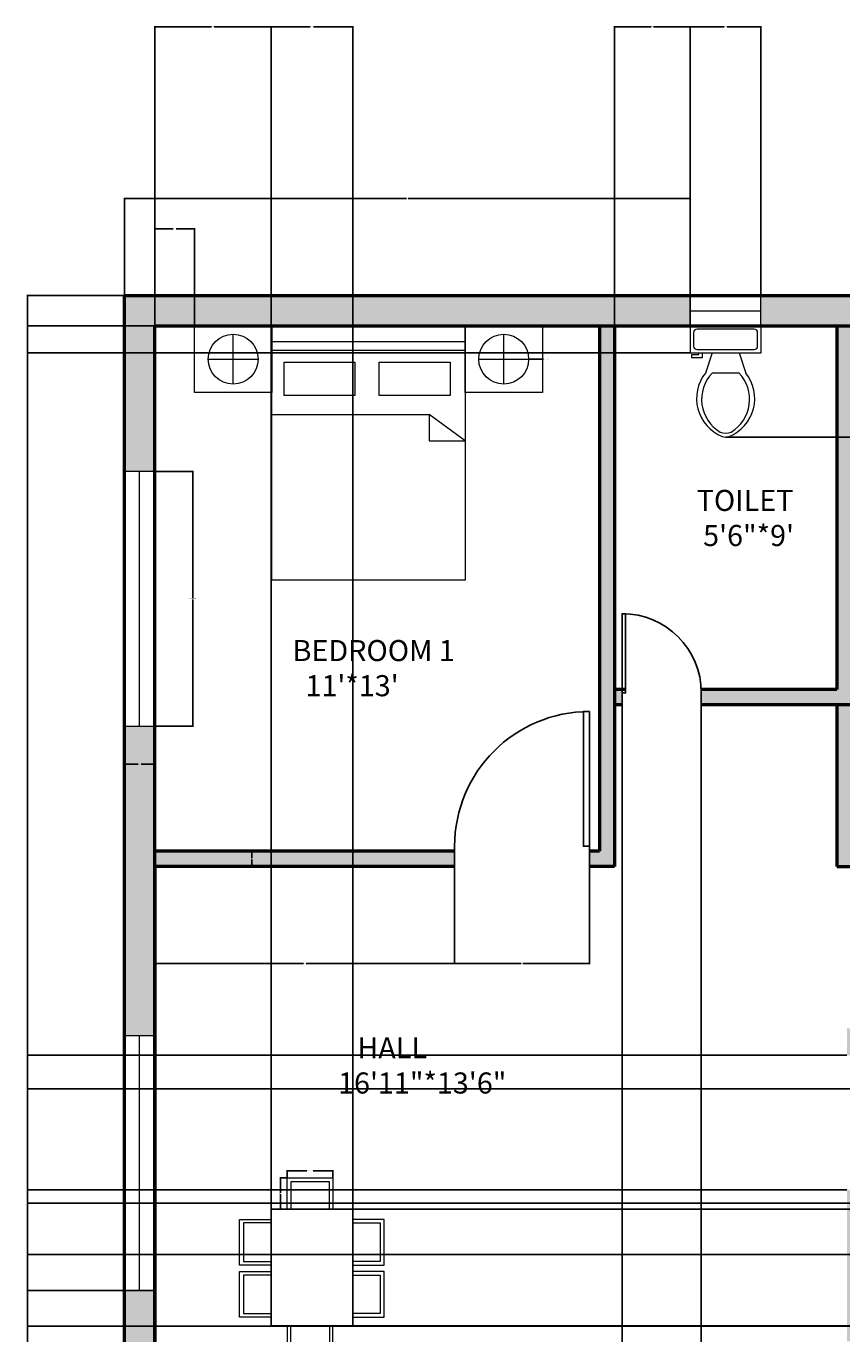
# Model space of a CAD drawing. Units: inches. Extents: x 2405 to 2823, y 1214 to 1813.
# Tile 3 of 4: x 2405 to 2647, y 1425 to 1813. Entities that reach past the tile are written whole.
import ezdxf

# ---------------------------------------------------------------- set-up
doc = ezdxf.new("R2010")
doc.units = ezdxf.units.IN
for name, color, linetype, lineweight in [('A-ANNO-DIMS', 2, 'Continuous', 18), ('A-AREA-IDEN', 30, 'Continuous', 25), ('A-FLOR-FIXT', 9, 'Continuous', 18), ('A-WALL-PATT', 252, 'Continuous', 13), ('DOOR', 133, 'Continuous', 25), ('FUR', 10, 'Continuous', 18), ('WALL', 140, 'Continuous', 50), ('WIND', 200, 'Continuous', 18)]:
    doc.layers.add(name, color=color, linetype=linetype, lineweight=lineweight)
doc.styles.get("Standard").update_dxf_attribs({"font": 'arial.ttf'})
doc.dimstyles.get("Standard").update_dxf_attribs({"dimtxt": 0.18, "dimasz": 0.18, "dimexe": 0.18, "dimexo": 0.0625, "dimgap": 0.09, "dimtad": 0, "dimtih": 1, "dimtoh": 1, "dimdec": 4, "dimzin": 0, "dimdsep": 46, "dimtxsty": 'Standard', "dimcen": 0.09, "dimadec": 0, "dimazin": 0, "dimtfac": 1, "dimtdec": 4, "dimtofl": 0, "dimtmove": 0, "dimatfit": 3, "dimfxl": 1, "dimtolj": 1, "dimtzin": 0, "dimarcsym": 0})

# ---------------------------------------------------------------- blocks, each defined once
blk = doc.blocks.new('*U2')
for p, q in [((0, 0), (0, -6)), ((40, 0), (40, -6))]:
    blk.add_line(p, q)
blk.add_lwpolyline([(0, 0), (0, 40), (1.75, 40), (1.75, 0)], close=True)
blk.add_arc((0, 0), 40, 0, 90)
blk = doc.blocks.new('*U4')
for p, q in [((9.5, -6), (9.5, -2)), ((-10, -8.5), (-8, -8.5)), ((-10, -9.5), (-10, -8.5)), ((-7, -9.5), (-10, -9.5)), ((-8, -8.5), (-8, -8)), ((-7, -8), (-7, -9.5)), ((-4, -8), (-6, -14)), ((4, -8), (6, -14)), ((4, -14), (-4, -14))]:
    blk.add_line(p, q)
blk.add_lwpolyline([(10.5, -8), (10.5, 0), (-10.5, 0), (-10.5, -8)], close=True)
for points in [[(-9.5, -2), (-9.5, -6)], [(8.5, -1), (-8.5, -1)], [(-8.5, -7), (8.5, -7)]]:
    blk.add_lwpolyline(points)
for centre, radius, start, end in [((-8.62, -1.88), 0.884, 81.8699, 188.1301), ((8.62, -1.88), 0.884, 351.8699, 98.1301), ((-8.62, -6.12), 0.884, 171.8699, 278.1301), ((8.62, -6.12), 0.884, 261.8699, 8.1301), ((3.52, -21.58), 12.17, 141.4691, 247.9714), ((4.2, -21.82), 11.33, 136.3677, 238.9468), ((-3.52, -21.58), 12.17, 292.0284, 38.5307), ((-4.2, -21.82), 11.33, 301.053, 43.6321), ((0, -27.88), 4, 245.7318, 294.2682), ((0, -29), 4, 254.8605, 285.1395)]:
    blk.add_arc(centre, radius, start, end)
blk = doc.blocks.new('BED-DOUBLE-WITH-NIGHTSTANDS')
for p, q in [((11.49, 58.17), (11.49, 72.97)), ((91.81, 58.17), (91.81, 72.97)), ((4.09, 65.57), (18.88, 65.57)), ((84.41, 65.57), (99.2, 65.57)), ((22.97, 49.14), (69.63, 49.14)), ((69.63, 49.14), (69.63, 41.32)), ((80.32, 41.32), (69.63, 49.14)), ((69.63, 41.32), (80.32, 41.32))]:
    blk.add_line(p, q)
for points in [[(0, 75.45), (22.97, 75.45), (22.97, 55.69), (0, 55.69)], [(22.97, 75.45), (80.32, 75.45), (80.32, 0), (22.97, 0)], [(80.32, 75.45), (103.29, 75.45), (103.29, 55.69), (80.32, 55.69)], [(22.97, 70.85), (80.32, 70.85), (80.32, 68.18), (22.97, 68.18)], [(26.59, 64.68), (47.64, 64.68), (47.64, 54.75), (26.59, 54.75)], [(54.85, 64.68), (75.89, 64.68), (75.89, 54.75), (54.85, 54.75)]]:
    blk.add_lwpolyline(points, close=True)
for centre in [(11.49, 65.57), (91.81, 65.57)]:
    blk.add_circle(centre, 7.4)
blk = doc.blocks.new('CHAIR-DINING')
for p, q in [((0, 0), (0, 9.36)), ((0, 9.36), (13.56, 9.36)), ((13.56, 9.36), (13.56, 0))]:
    blk.add_line(p, q)
blk.add_lwpolyline([(1.08, 0), (12.53, 0), (12.53, 8.17), (1.08, 8.17)], close=True)
blk = doc.blocks.new('WIN-75_625')
blk.add_line((4.5, 0), (4.5, 75.63))
blk.add_lwpolyline([(9, 75.63), (0, 75.63), (0, 0), (9, 0)], close=True)
blk = doc.blocks.new('*D12')
at = {"layer": 'A-ANNO-DIMS', "color": 0, "lineweight": -2, "transparency": 16777216}
for p, q in [((2482.12, 1471.1), (2482.12, 1473.25)), ((2482.3, 1473.07), (2487.95, 1473.07)), ((2495.5, 1473.07), (2489.85, 1473.07)), ((2495.68, 1471.1), (2495.68, 1473.25))]:
    blk.add_line(p, q, dxfattribs=at)
at = {"layer": 'A-ANNO-DIMS', "color": 0, "lineweight": 100, "transparency": 16777216}
for points in [[(2482.3, 1473.1), (2482.3, 1473.04), (2482.12, 1473.07)], [(2495.5, 1473.1), (2495.5, 1473.04), (2495.68, 1473.07)]]:
    blk.add_solid(points, dxfattribs=at)
at = {"layer": 'Defpoints', "color": 0, "lineweight": 100, "transparency": 16777216}
for p in [(2495.68, 1473.07), (2482.12, 1471.04), (2495.68, 1471.04)]:
    blk.add_point(p, dxfattribs=at)
at = {"layer": 'A-ANNO-DIMS', "color": 0, "transparency": 16777216, "insert": (2488.9, 1473.07), "char_height": 0.18, "attachment_point": 5}
blk.add_mtext('\\A1;CHAIR 14 TYP.', dxfattribs=at)
blk = doc.blocks.new('*D13')
at = {"layer": 'A-ANNO-DIMS', "color": 0, "lineweight": -2, "transparency": 16777216}
for p, q in [((2482.06, 1471.04), (2479.9, 1471.04)), ((2480.08, 1470.86), (2480.08, 1466.54)), ((2480.08, 1461.86), (2480.08, 1466.17)), ((2482.06, 1461.68), (2479.9, 1461.68))]:
    blk.add_line(p, q, dxfattribs=at)
at = {"layer": 'A-ANNO-DIMS', "color": 0, "lineweight": 100, "transparency": 16777216}
for points in [[(2480.05, 1470.86), (2480.11, 1470.86), (2480.08, 1471.04)], [(2480.05, 1461.86), (2480.11, 1461.86), (2480.08, 1461.68)]]:
    blk.add_solid(points, dxfattribs=at)
at = {"layer": 'Defpoints', "color": 0, "lineweight": 100, "transparency": 16777216}
for p in [(2480.08, 1471.04), (2482.12, 1471.04), (2482.12, 1461.68)]:
    blk.add_point(p, dxfattribs=at)
at = {"layer": 'A-ANNO-DIMS', "color": 0, "transparency": 16777216, "insert": (2480.08, 1466.36), "char_height": 0.18, "attachment_point": 5}
blk.add_mtext('\\A1;9 TYP.', dxfattribs=at)
blk = doc.blocks.new('*D18')
at = {"layer": 'A-ANNO-DIMS', "color": 0, "lineweight": -2, "transparency": 16777216}
for p, q in [((2442.83, 1680.74), (2454.29, 1680.74)), ((2454.11, 1680.56), (2454.11, 1643.11)), ((2454.11, 1605.29), (2454.11, 1642.74)), ((2442.83, 1605.11), (2454.29, 1605.11))]:
    blk.add_line(p, q, dxfattribs=at)
at = {"layer": 'A-ANNO-DIMS', "color": 0, "lineweight": 100, "transparency": 16777216}
for points in [[(2454.08, 1680.56), (2454.14, 1680.56), (2454.11, 1680.74)], [(2454.08, 1605.29), (2454.14, 1605.29), (2454.11, 1605.11)]]:
    blk.add_solid(points, dxfattribs=at)
at = {"layer": 'Defpoints', "color": 0, "lineweight": 100, "transparency": 16777216}
for p in [(2442.77, 1680.74), (2454.11, 1680.74), (2442.77, 1605.11)]:
    blk.add_point(p, dxfattribs=at)
at = {"layer": 'A-ANNO-DIMS', "color": 0, "transparency": 16777216, "insert": (2454.11, 1642.92), "char_height": 0.18, "attachment_point": 5}
blk.add_mtext('\\A1;WINDOW 76 TYP.', dxfattribs=at)
blk = doc.blocks.new('*D19')
at = {"layer": 'A-ANNO-DIMS', "color": 0, "lineweight": -2, "transparency": 16777216}
for p, q in [((2433.77, 1605.05), (2433.77, 1593.59)), ((2442.77, 1605.05), (2442.77, 1593.59)), ((2433.95, 1593.77), (2437.81, 1593.77)), ((2442.59, 1593.77), (2438.73, 1593.77))]:
    blk.add_line(p, q, dxfattribs=at)
at = {"layer": 'A-ANNO-DIMS', "color": 0, "lineweight": 100, "transparency": 16777216}
for points in [[(2433.95, 1593.8), (2433.95, 1593.74), (2433.77, 1593.77)], [(2442.59, 1593.8), (2442.59, 1593.74), (2442.77, 1593.77)]]:
    blk.add_solid(points, dxfattribs=at)
at = {"layer": 'Defpoints', "color": 0, "lineweight": 100, "transparency": 16777216}
for p in [(2433.77, 1605.11), (2442.77, 1605.11), (2442.77, 1593.77)]:
    blk.add_point(p, dxfattribs=at)
at = {"layer": 'A-ANNO-DIMS', "color": 0, "transparency": 16777216, "insert": (2438.27, 1593.77), "char_height": 0.18, "attachment_point": 5}
blk.add_mtext('\\A1;9 TYP.', dxfattribs=at)
blk = doc.blocks.new('*D23')
at = {"layer": 'A-ANNO-DIMS', "color": 0, "lineweight": -2, "transparency": 16777216}
for p, q in [((2433.71, 1732.93), (2404.79, 1732.93)), ((2404.97, 1732.75), (2404.97, 1488.61)), ((2404.97, 1244.11), (2404.97, 1488.25)), ((2586.21, 1243.93), (2404.79, 1243.93))]:
    blk.add_line(p, q, dxfattribs=at)
at = {"layer": 'A-ANNO-DIMS', "color": 0, "lineweight": 100, "transparency": 16777216}
for points in [[(2404.94, 1732.75), (2405, 1732.75), (2404.97, 1732.93)], [(2404.94, 1244.11), (2405, 1244.11), (2404.97, 1243.93)]]:
    blk.add_solid(points, dxfattribs=at)
at = {"layer": 'Defpoints', "color": 0, "lineweight": 100, "transparency": 16777216}
for p in [(2433.77, 1732.93), (2404.97, 1243.93), (2586.27, 1243.93)]:
    blk.add_point(p, dxfattribs=at)
at = {"layer": 'A-ANNO-DIMS', "color": 0, "transparency": 16777216, "insert": (2404.97, 1488.43), "char_height": 0.18, "attachment_point": 5}
blk.add_mtext('\\A1;489', dxfattribs=at)
blk = doc.blocks.new('*D25')
at = {"layer": 'A-ANNO-DIMS', "color": 0, "lineweight": -2, "transparency": 16777216}
for p, q in [((2442.71, 1437.52), (2404.79, 1437.52)), ((2404.97, 1437.34), (2404.97, 1419.66)), ((2404.97, 1401.61), (2404.97, 1419.29)), ((2442.71, 1401.43), (2404.79, 1401.43))]:
    blk.add_line(p, q, dxfattribs=at)
at = {"layer": 'A-ANNO-DIMS', "color": 0, "lineweight": 100, "transparency": 16777216}
for points in [[(2404.94, 1437.34), (2405, 1437.34), (2404.97, 1437.52)], [(2404.94, 1401.61), (2405, 1401.61), (2404.97, 1401.43)]]:
    blk.add_solid(points, dxfattribs=at)
at = {"layer": 'Defpoints', "color": 0, "lineweight": 100, "transparency": 16777216}
for p in [(2442.77, 1437.52), (2404.97, 1401.43), (2442.77, 1401.43)]:
    blk.add_point(p, dxfattribs=at)
at = {"layer": 'A-ANNO-DIMS', "color": 0, "transparency": 16777216, "insert": (2404.97, 1419.47), "char_height": 0.18, "attachment_point": 5}
blk.add_mtext('\\A1;36.09', dxfattribs=at)
blk = doc.blocks.new('*D32')
at = {"layer": 'A-ANNO-DIMS', "color": 0, "lineweight": -2, "transparency": 16777216}
for p, q in [((2433.77, 1732.99), (2433.77, 1761.91)), ((2433.95, 1761.73), (2517.49, 1761.73)), ((2601.59, 1761.73), (2518.05, 1761.73)), ((2601.77, 1732.99), (2601.77, 1761.91))]:
    blk.add_line(p, q, dxfattribs=at)
at = {"layer": 'A-ANNO-DIMS', "color": 0, "lineweight": 100, "transparency": 16777216}
for points in [[(2433.95, 1761.76), (2433.95, 1761.7), (2433.77, 1761.73)], [(2601.59, 1761.76), (2601.59, 1761.7), (2601.77, 1761.73)]]:
    blk.add_solid(points, dxfattribs=at)
at = {"layer": 'Defpoints', "color": 0, "lineweight": 100, "transparency": 16777216}
for p in [(2601.77, 1761.73), (2433.77, 1732.93), (2601.77, 1732.93)]:
    blk.add_point(p, dxfattribs=at)
at = {"layer": 'A-ANNO-DIMS', "color": 0, "transparency": 16777216, "insert": (2517.77, 1761.73), "char_height": 0.18, "attachment_point": 5}
blk.add_mtext('\\A1;168', dxfattribs=at)
blk = doc.blocks.new('*D33')
at = {"layer": 'A-ANNO-DIMS', "color": 0, "lineweight": -2, "transparency": 16777216}
for p, q in [((2601.77, 1732.99), (2601.77, 1812.91)), ((2601.95, 1812.73), (2611.8, 1812.73)), ((2622.58, 1812.73), (2612.73, 1812.73)), ((2622.76, 1732.99), (2622.76, 1812.91))]:
    blk.add_line(p, q, dxfattribs=at)
at = {"layer": 'A-ANNO-DIMS', "color": 0, "lineweight": 100, "transparency": 16777216}
for points in [[(2601.95, 1812.76), (2601.95, 1812.7), (2601.77, 1812.73)], [(2622.58, 1812.76), (2622.58, 1812.7), (2622.76, 1812.73)]]:
    blk.add_solid(points, dxfattribs=at)
at = {"layer": 'Defpoints', "color": 0, "lineweight": 100, "transparency": 16777216}
for p in [(2622.76, 1812.73), (2601.77, 1732.93), (2622.76, 1732.93)]:
    blk.add_point(p, dxfattribs=at)
at = {"layer": 'A-ANNO-DIMS', "color": 0, "transparency": 16777216, "insert": (2612.26, 1812.73), "char_height": 0.18, "attachment_point": 5}
blk.add_mtext('\\A1;20.987', dxfattribs=at)
blk = doc.blocks.new('*D41')
at = {"layer": 'A-ANNO-DIMS', "color": 0, "lineweight": -2, "transparency": 16777216}
for p, q in [((2648.21, 1507.39), (2404.79, 1507.39)), ((2404.97, 1507.21), (2404.97, 1487.57)), ((2404.97, 1467.57), (2404.97, 1487.21)), ((2648.21, 1467.39), (2404.79, 1467.39))]:
    blk.add_line(p, q, dxfattribs=at)
at = {"layer": 'A-ANNO-DIMS', "color": 0, "lineweight": 100, "transparency": 16777216}
for points in [[(2404.94, 1507.21), (2405, 1507.21), (2404.97, 1507.39)], [(2404.94, 1467.57), (2405, 1467.57), (2404.97, 1467.39)]]:
    blk.add_solid(points, dxfattribs=at)
at = {"layer": 'Defpoints', "color": 0, "lineweight": 100, "transparency": 16777216}
for p in [(2648.27, 1507.39), (2404.97, 1467.39), (2648.27, 1467.39)]:
    blk.add_point(p, dxfattribs=at)
at = {"layer": 'A-ANNO-DIMS', "color": 0, "transparency": 16777216, "insert": (2404.97, 1487.39), "char_height": 0.18, "attachment_point": 5}
blk.add_mtext('\\A1;40', dxfattribs=at)
blk = doc.blocks.new('*D42')
at = {"layer": 'A-ANNO-DIMS', "color": 0, "lineweight": -2, "transparency": 16777216}
for p, q in [((2605.03, 1615.87), (2605.03, 1214.95)), ((2581.53, 1614.9), (2581.53, 1214.95)), ((2581.71, 1215.13), (2592.95, 1215.13)), ((2604.85, 1215.13), (2593.61, 1215.13))]:
    blk.add_line(p, q, dxfattribs=at)
at = {"layer": 'A-ANNO-DIMS', "color": 0, "lineweight": 100, "transparency": 16777216}
for points in [[(2581.71, 1215.16), (2581.71, 1215.1), (2581.53, 1215.13)], [(2604.85, 1215.16), (2604.85, 1215.1), (2605.03, 1215.13)]]:
    blk.add_solid(points, dxfattribs=at)
at = {"layer": 'Defpoints', "color": 0, "lineweight": 100, "transparency": 16777216}
for p in [(2605.03, 1615.93), (2581.53, 1614.96), (2605.03, 1215.13)]:
    blk.add_point(p, dxfattribs=at)
at = {"layer": 'A-ANNO-DIMS', "color": 0, "transparency": 16777216, "insert": (2593.28, 1215.13), "char_height": 0.18, "attachment_point": 5}
blk.add_mtext('\\A1;23.5', dxfattribs=at)
blk = doc.blocks.new('*D44')
at = {"layer": 'A-ANNO-DIMS', "color": 0, "lineweight": -2, "transparency": 16777216}
for p, q in [((2477.3, 1427.08), (2477.3, 1812.91)), ((2477.48, 1812.73), (2488.96, 1812.73)), ((2501.38, 1812.73), (2489.89, 1812.73)), ((2501.56, 1427.08), (2501.56, 1812.91))]:
    blk.add_line(p, q, dxfattribs=at)
at = {"layer": 'A-ANNO-DIMS', "color": 0, "lineweight": 100, "transparency": 16777216}
for points in [[(2477.48, 1812.76), (2477.48, 1812.7), (2477.3, 1812.73)], [(2501.38, 1812.76), (2501.38, 1812.7), (2501.56, 1812.73)]]:
    blk.add_solid(points, dxfattribs=at)
at = {"layer": 'Defpoints', "color": 0, "lineweight": 100, "transparency": 16777216}
for p in [(2501.56, 1812.73), (2477.3, 1427.01), (2501.56, 1427.01)]:
    blk.add_point(p, dxfattribs=at)
at = {"layer": 'A-ANNO-DIMS', "color": 0, "transparency": 16777216, "insert": (2489.43, 1812.73), "char_height": 0.18, "attachment_point": 5}
blk.add_mtext('\\A1;24.266', dxfattribs=at)
blk = doc.blocks.new('*D45')
at = {"layer": 'A-ANNO-DIMS', "color": 0, "lineweight": -2, "transparency": 16777216}
for p, q in [((2477.36, 1461.68), (2822.75, 1461.68)), ((2822.57, 1461.5), (2822.57, 1444.53)), ((2822.57, 1427.19), (2822.57, 1444.16)), ((2477.36, 1427.01), (2822.75, 1427.01))]:
    blk.add_line(p, q, dxfattribs=at)
at = {"layer": 'A-ANNO-DIMS', "color": 0, "lineweight": 100, "transparency": 16777216}
for points in [[(2822.54, 1461.5), (2822.6, 1461.5), (2822.57, 1461.68)], [(2822.54, 1427.19), (2822.6, 1427.19), (2822.57, 1427.01)]]:
    blk.add_solid(points, dxfattribs=at)
at = {"layer": 'Defpoints', "color": 0, "lineweight": 100, "transparency": 16777216}
for p in [(2477.3, 1461.68), (2477.3, 1427.01), (2822.57, 1427.01)]:
    blk.add_point(p, dxfattribs=at)
at = {"layer": 'A-ANNO-DIMS', "color": 0, "transparency": 16777216, "insert": (2822.57, 1444.34), "char_height": 0.18, "attachment_point": 5}
blk.add_mtext('\\A1;34.66', dxfattribs=at)
blk = doc.blocks.new('*D47')
at = {"layer": 'A-ANNO-DIMS', "color": 0, "lineweight": -2, "transparency": 16777216}
for p, q in [((2763.89, 1497.45), (2404.79, 1497.45)), ((2404.97, 1497.27), (2404.97, 1480.64)), ((2404.97, 1463.65), (2404.97, 1480.28)), ((2763.89, 1463.47), (2404.79, 1463.47))]:
    blk.add_line(p, q, dxfattribs=at)
at = {"layer": 'A-ANNO-DIMS', "color": 0, "lineweight": 100, "transparency": 16777216}
for points in [[(2404.94, 1497.27), (2405, 1497.27), (2404.97, 1497.45)], [(2404.94, 1463.65), (2405, 1463.65), (2404.97, 1463.47)]]:
    blk.add_solid(points, dxfattribs=at)
at = {"layer": 'Defpoints', "color": 0, "lineweight": 100, "transparency": 16777216}
for p in [(2763.95, 1497.45), (2404.97, 1463.47), (2763.95, 1463.47)]:
    blk.add_point(p, dxfattribs=at)
at = {"layer": 'A-ANNO-DIMS', "color": 0, "transparency": 16777216, "insert": (2404.97, 1480.46), "char_height": 0.18, "attachment_point": 5}
blk.add_mtext('\\A1;33.98', dxfattribs=at)
blk = doc.blocks.new('*D49')
at = {"layer": 'A-ANNO-DIMS', "color": 0, "lineweight": -2, "transparency": 16777216}
for p, q in [((2442.77, 1401.49), (2442.77, 1812.91)), ((2442.95, 1812.73), (2459.64, 1812.73)), ((2477.12, 1812.73), (2460.43, 1812.73)), ((2477.3, 1427.08), (2477.3, 1812.91))]:
    blk.add_line(p, q, dxfattribs=at)
at = {"layer": 'A-ANNO-DIMS', "color": 0, "lineweight": 100, "transparency": 16777216}
for points in [[(2442.95, 1812.76), (2442.95, 1812.7), (2442.77, 1812.73)], [(2477.12, 1812.76), (2477.12, 1812.7), (2477.3, 1812.73)]]:
    blk.add_solid(points, dxfattribs=at)
at = {"layer": 'Defpoints', "color": 0, "lineweight": 100, "transparency": 16777216}
for p in [(2477.3, 1812.73), (2477.3, 1427.01), (2442.77, 1401.43)]:
    blk.add_point(p, dxfattribs=at)
at = {"layer": 'A-ANNO-DIMS', "color": 0, "transparency": 16777216, "insert": (2460.03, 1812.73), "char_height": 0.18, "attachment_point": 5}
blk.add_mtext('\\A1;34.53', dxfattribs=at)
blk = doc.blocks.new('*D50')
at = {"layer": 'A-ANNO-DIMS', "color": 0, "lineweight": -2, "transparency": 16777216}
for p, q in [((2477.36, 1427.01), (2822.75, 1427.01)), ((2822.57, 1426.83), (2822.57, 1414.4)), ((2822.57, 1401.61), (2822.57, 1414.04)), ((2442.83, 1401.43), (2822.75, 1401.43))]:
    blk.add_line(p, q, dxfattribs=at)
at = {"layer": 'A-ANNO-DIMS', "color": 0, "lineweight": 100, "transparency": 16777216}
for points in [[(2822.54, 1426.83), (2822.6, 1426.83), (2822.57, 1427.01)], [(2822.54, 1401.61), (2822.6, 1401.61), (2822.57, 1401.43)]]:
    blk.add_solid(points, dxfattribs=at)
at = {"layer": 'Defpoints', "color": 0, "lineweight": 100, "transparency": 16777216}
for p in [(2477.3, 1427.01), (2822.57, 1427.01), (2442.77, 1401.43)]:
    blk.add_point(p, dxfattribs=at)
at = {"layer": 'A-ANNO-DIMS', "color": 0, "transparency": 16777216, "insert": (2822.57, 1414.22), "char_height": 0.18, "attachment_point": 5}
blk.add_mtext('\\A1;25.584', dxfattribs=at)
blk = doc.blocks.new('*D52')
at = {"layer": 'A-ANNO-DIMS', "color": 0, "lineweight": -2, "transparency": 16777216}
for p, q in [((2442.77, 1723.99), (2442.77, 1752.91)), ((2442.95, 1752.73), (2448.21, 1752.73)), ((2454.39, 1752.73), (2449.12, 1752.73)), ((2454.57, 1723.99), (2454.57, 1752.91))]:
    blk.add_line(p, q, dxfattribs=at)
at = {"layer": 'A-ANNO-DIMS', "color": 0, "lineweight": 100, "transparency": 16777216}
for points in [[(2442.95, 1752.76), (2442.95, 1752.7), (2442.77, 1752.73)], [(2454.39, 1752.76), (2454.39, 1752.7), (2454.57, 1752.73)]]:
    blk.add_solid(points, dxfattribs=at)
at = {"layer": 'Defpoints', "color": 0, "lineweight": 100, "transparency": 16777216}
for p in [(2454.57, 1752.73), (2442.77, 1723.93), (2454.57, 1723.93)]:
    blk.add_point(p, dxfattribs=at)
at = {"layer": 'A-ANNO-DIMS', "color": 0, "transparency": 16777216, "insert": (2448.67, 1752.73), "char_height": 0.18, "attachment_point": 5}
blk.add_mtext('\\A1;11.802', dxfattribs=at)
blk = doc.blocks.new('*D56')
at = {"layer": 'A-ANNO-DIMS', "color": 0, "lineweight": -2, "transparency": 16777216}
for p, q in [((2442.83, 1567.93), (2471.75, 1567.93)), ((2471.57, 1567.75), (2471.57, 1565.86)), ((2471.57, 1563.61), (2471.57, 1565.5)), ((2442.83, 1563.43), (2471.75, 1563.43))]:
    blk.add_line(p, q, dxfattribs=at)
at = {"layer": 'A-ANNO-DIMS', "color": 0, "lineweight": 100, "transparency": 16777216}
for points in [[(2471.54, 1567.75), (2471.6, 1567.75), (2471.57, 1567.93)], [(2471.54, 1563.61), (2471.6, 1563.61), (2471.57, 1563.43)]]:
    blk.add_solid(points, dxfattribs=at)
at = {"layer": 'Defpoints', "color": 0, "lineweight": 100, "transparency": 16777216}
for p in [(2442.77, 1567.93), (2442.77, 1563.43), (2471.57, 1563.43)]:
    blk.add_point(p, dxfattribs=at)
at = {"layer": 'A-ANNO-DIMS', "color": 0, "transparency": 16777216, "insert": (2471.57, 1565.68), "char_height": 0.18, "attachment_point": 5}
blk.add_mtext('\\A1;4.5', dxfattribs=at)
blk = doc.blocks.new('*D57')
at = {"layer": 'A-ANNO-DIMS', "color": 0, "lineweight": -2, "transparency": 16777216}
for p, q in [((2622.83, 1723.93), (2822.75, 1723.93)), ((2822.57, 1723.75), (2822.57, 1707.61)), ((2822.57, 1691.11), (2822.57, 1707.25)), ((2612.33, 1690.93), (2822.75, 1690.93))]:
    blk.add_line(p, q, dxfattribs=at)
at = {"layer": 'A-ANNO-DIMS', "color": 0, "lineweight": 100, "transparency": 16777216}
for points in [[(2822.54, 1723.75), (2822.6, 1723.75), (2822.57, 1723.93)], [(2822.54, 1691.11), (2822.6, 1691.11), (2822.57, 1690.93)]]:
    blk.add_solid(points, dxfattribs=at)
at = {"layer": 'Defpoints', "color": 0, "lineweight": 100, "transparency": 16777216}
for p in [(2622.77, 1723.93), (2612.27, 1690.93), (2822.57, 1690.93)]:
    blk.add_point(p, dxfattribs=at)
at = {"layer": 'A-ANNO-DIMS', "color": 0, "transparency": 16777216, "insert": (2822.57, 1707.43), "char_height": 0.18, "attachment_point": 5}
blk.add_mtext('\\A1;33', dxfattribs=at)
blk = doc.blocks.new('*D62')
at = {"layer": 'A-ANNO-DIMS', "color": 0, "lineweight": -2, "transparency": 16777216}
for p, q in [((2579.27, 1723.99), (2579.27, 1812.91)), ((2579.45, 1812.73), (2590.19, 1812.73)), ((2601.59, 1812.73), (2590.84, 1812.73)), ((2601.77, 1723.99), (2601.77, 1812.91))]:
    blk.add_line(p, q, dxfattribs=at)
at = {"layer": 'A-ANNO-DIMS', "color": 0, "lineweight": 100, "transparency": 16777216}
for points in [[(2579.45, 1812.76), (2579.45, 1812.7), (2579.27, 1812.73)], [(2601.59, 1812.76), (2601.59, 1812.7), (2601.77, 1812.73)]]:
    blk.add_solid(points, dxfattribs=at)
at = {"layer": 'Defpoints', "color": 0, "lineweight": 100, "transparency": 16777216}
for p in [(2601.77, 1812.73), (2579.27, 1723.93), (2601.77, 1723.93)]:
    blk.add_point(p, dxfattribs=at)
at = {"layer": 'A-ANNO-DIMS', "color": 0, "transparency": 16777216, "insert": (2590.52, 1812.73), "char_height": 0.18, "attachment_point": 5}
blk.add_mtext('\\A1;22.5', dxfattribs=at)
blk = doc.blocks.new('*D63')
at = {"layer": 'A-ANNO-DIMS', "color": 0, "lineweight": -2, "transparency": 16777216}
for p, q in [((2601.71, 1723.93), (2404.79, 1723.93)), ((2404.97, 1723.75), (2404.97, 1720.11)), ((2404.97, 1716.11), (2404.97, 1719.75)), ((2601.71, 1715.93), (2404.79, 1715.93))]:
    blk.add_line(p, q, dxfattribs=at)
at = {"layer": 'A-ANNO-DIMS', "color": 0, "lineweight": 100, "transparency": 16777216}
for points in [[(2404.94, 1723.75), (2405, 1723.75), (2404.97, 1723.93)], [(2404.94, 1716.11), (2405, 1716.11), (2404.97, 1715.93)]]:
    blk.add_solid(points, dxfattribs=at)
at = {"layer": 'Defpoints', "color": 0, "lineweight": 100, "transparency": 16777216}
for p in [(2601.77, 1723.93), (2404.97, 1715.93), (2601.77, 1715.93)]:
    blk.add_point(p, dxfattribs=at)
at = {"layer": 'A-ANNO-DIMS', "color": 0, "transparency": 16777216, "insert": (2404.97, 1719.93), "char_height": 0.18, "attachment_point": 5}
blk.add_mtext('\\A1;8', dxfattribs=at)
blk = doc.blocks.new('*D64')
at = {"layer": 'A-ANNO-DIMS', "color": 0, "lineweight": -2, "transparency": 16777216}
for p, q in [((2442.77, 1563.37), (2442.77, 1534.45)), ((2531.81, 1563.37), (2531.81, 1534.45)), ((2442.95, 1534.63), (2486.89, 1534.63)), ((2531.63, 1534.63), (2487.68, 1534.63))]:
    blk.add_line(p, q, dxfattribs=at)
at = {"layer": 'A-ANNO-DIMS', "color": 0, "lineweight": 100, "transparency": 16777216}
for points in [[(2442.95, 1534.66), (2442.95, 1534.6), (2442.77, 1534.63)], [(2531.63, 1534.66), (2531.63, 1534.6), (2531.81, 1534.63)]]:
    blk.add_solid(points, dxfattribs=at)
at = {"layer": 'Defpoints', "color": 0, "lineweight": 100, "transparency": 16777216}
for p in [(2442.77, 1563.43), (2531.81, 1563.43), (2442.77, 1534.63)]:
    blk.add_point(p, dxfattribs=at)
at = {"layer": 'A-ANNO-DIMS', "color": 0, "transparency": 16777216, "insert": (2487.29, 1534.63), "char_height": 0.18, "attachment_point": 5}
blk.add_mtext('\\A1;89.04', dxfattribs=at)
blk = doc.blocks.new('*D65')
at = {"layer": 'A-ANNO-DIMS', "color": 0, "lineweight": -2, "transparency": 16777216}
for p, q in [((2531.81, 1563.37), (2531.81, 1534.45)), ((2571.81, 1563.37), (2571.81, 1534.45)), ((2531.99, 1534.63), (2551.58, 1534.63)), ((2571.63, 1534.63), (2552.03, 1534.63))]:
    blk.add_line(p, q, dxfattribs=at)
at = {"layer": 'A-ANNO-DIMS', "color": 0, "lineweight": 100, "transparency": 16777216}
for points in [[(2531.99, 1534.66), (2531.99, 1534.6), (2531.81, 1534.63)], [(2571.63, 1534.66), (2571.63, 1534.6), (2571.81, 1534.63)]]:
    blk.add_solid(points, dxfattribs=at)
at = {"layer": 'Defpoints', "color": 0, "lineweight": 100, "transparency": 16777216}
for p in [(2531.81, 1563.43), (2571.81, 1563.43), (2531.81, 1534.63)]:
    blk.add_point(p, dxfattribs=at)
at = {"layer": 'A-ANNO-DIMS', "color": 0, "transparency": 16777216, "insert": (2551.81, 1534.63), "char_height": 0.18, "attachment_point": 5}
blk.add_mtext('\\A1;40', dxfattribs=at)
blk = doc.blocks.new('*D68')
at = {"layer": 'A-ANNO-DIMS', "color": 0, "lineweight": -2, "transparency": 16777216}
for p, q in [((2688.36, 1448.27), (2404.79, 1448.27)), ((2404.97, 1448.09), (2404.97, 1437.78)), ((2404.97, 1427.11), (2404.97, 1437.42)), ((2688.36, 1426.93), (2404.79, 1426.93))]:
    blk.add_line(p, q, dxfattribs=at)
at = {"layer": 'A-ANNO-DIMS', "color": 0, "lineweight": 100, "transparency": 16777216}
for points in [[(2404.94, 1448.09), (2405, 1448.09), (2404.97, 1448.27)], [(2404.94, 1427.11), (2405, 1427.11), (2404.97, 1426.93)]]:
    blk.add_solid(points, dxfattribs=at)
at = {"layer": 'Defpoints', "color": 0, "lineweight": 100, "transparency": 16777216}
for p in [(2688.42, 1448.27), (2404.97, 1426.93), (2688.42, 1426.93)]:
    blk.add_point(p, dxfattribs=at)
at = {"layer": 'A-ANNO-DIMS', "color": 0, "transparency": 16777216, "insert": (2404.97, 1437.6), "char_height": 0.18, "attachment_point": 5}
blk.add_mtext('\\A1;21.336', dxfattribs=at)
blk = doc.blocks.new('*D71')
at = {"layer": 'A-ANNO-DIMS', "color": 0, "lineweight": -2, "transparency": 16777216}
for p, q in [((2546.29, 1714.05), (2546.47, 1714.05)), ((2546.38, 1713.96), (2546.38, 1714.14)), ((2558.21, 1714.05), (2553.95, 1714.05))]:
    blk.add_line(p, q, dxfattribs=at)
at = {"layer": 'A-ANNO-DIMS', "color": 0, "lineweight": 100, "transparency": 16777216}
blk.add_solid([(2553.95, 1714.08), (2553.95, 1714.02), (2553.77, 1714.05)], dxfattribs=at)
at = {"layer": 'Defpoints', "color": 0, "lineweight": 100, "transparency": 16777216}
for p in [(2538.98, 1714.05), (2553.77, 1714.05)]:
    blk.add_point(p, dxfattribs=at)
at = {"layer": 'A-ANNO-DIMS', "color": 0, "transparency": 16777216, "insert": (2558.96, 1714.05), "char_height": 0.18, "attachment_point": 5}
blk.add_mtext('\\A1;6X ∅14.797', dxfattribs=at)

msp = doc.modelspace()

# ---------------------------------------------------------------- hatches: boundary and pattern name
at = {"layer": 'A-WALL-PATT'}
h = msp.add_hatch(color=256, dxfattribs=at)
h.dxf.hatch_style = 1
h.paths.add_polyline_path([(2601.7679, 1732.9303), (2433.7679, 1732.9303), (2433.7679, 1680.7368), (2442.7679, 1680.7368), (2442.7679, 1723.9303), (2574.7679, 1723.9303), (2601.7679, 1723.9303)])
h.paths.add_polyline_path([(2793.7679, 1732.9303), (2622.7552, 1732.9303), (2622.7552, 1723.9303), (2622.7679, 1723.9303), (2645.2679, 1723.9303), (2784.7679, 1723.9303), (2784.7679, 1680.7368), (2793.7679, 1680.7368)])
h.paths.add_polyline_path([(2442.7679, 1605.111), (2433.7679, 1605.111), (2433.7679, 1513.1454), (2442.7679, 1513.1454), (2442.7679, 1563.4303)])
h.paths.add_polyline_path([(2531.8067, 1567.9303), (2442.7679, 1567.9303), (2442.7679, 1563.4303), (2531.8067, 1563.4303)])
h.paths.add_polyline_path([(2793.7679, 1605.111), (2784.7679, 1605.111), (2784.7679, 1555.6662), (2793.7679, 1555.6662)])
h.paths.add_polyline_path([(2784.7679, 1567.9303), (2691.5187, 1567.9303), (2691.5187, 1563.4303), (2784.7679, 1563.4303)])
h.paths.add_polyline_path([(2649.7679, 1611.4303), (2645.2679, 1611.4303), (2645.2679, 1563.4303), (2651.5187, 1563.4303), (2651.5187, 1567.9303), (2649.7679, 1567.9303)])
h.paths.add_polyline_path([(2581.5294, 1614.9584), (2581.5294, 1615.9303), (2579.2679, 1615.9303), (2579.2679, 1611.4303), (2581.5294, 1611.4303)])
h.paths.add_polyline_path([(2579.2679, 1723.9303), (2574.7679, 1723.9303), (2574.7679, 1567.9303), (2571.8067, 1567.9303), (2571.8067, 1563.4303), (2579.2679, 1563.4303)])
h.paths.add_polyline_path([(2649.7679, 1723.9303), (2645.2679, 1723.9303), (2645.2679, 1615.9303), (2605.0298, 1615.9303, -0.01033406), (2605.0499, 1614.9584), (2605.0499, 1611.4303), (2649.7679, 1611.4303)])
h.paths.add_polyline_path([(2793.7679, 1523.737), (2784.7679, 1523.737), (2784.7679, 1492.9303), (2793.7679, 1492.9303)])
h.paths.add_polyline_path([(2793.7679, 1446.4039), (2784.7679, 1446.4039), (2784.7679, 1426.9303), (2784.7679, 1412.6503), (2793.7679, 1412.6503)])
h.paths.add_polyline_path([(2652.7679, 1467.3906), (2648.2679, 1467.3906), (2648.2679, 1422.4303), (2784.7679, 1422.4303), (2784.7679, 1426.9303), (2652.7679, 1426.9303)])
h.paths.add_polyline_path([(2696.2679, 1515.4303), (2648.2679, 1515.4303), (2648.2679, 1507.3906), (2652.7679, 1507.3906), (2652.7679, 1510.9303), (2696.2679, 1510.9303)])
h.paths.add_polyline_path([(2784.7679, 1515.4303), (2700.7679, 1515.4303), (2696.2679, 1515.4303), (2696.2679, 1510.9303), (2784.7679, 1510.9303)])
h.paths.add_polyline_path([(2700.7679, 1522.7934), (2696.2679, 1522.7934), (2696.2679, 1515.4303), (2700.7679, 1515.4303)])
h.paths.add_polyline_path([(2700.7679, 1563.4303), (2696.2679, 1563.4303), (2696.2679, 1557.1044), (2700.7679, 1557.1044)])
h.paths.add_polyline_path([(2442.7679, 1437.5196), (2433.7679, 1437.5196), (2433.7679, 1252.9303), (2481.6786, 1252.9303), (2481.6786, 1261.9303), (2442.7679, 1261.9303)])
h.paths.add_polyline_path([(2536.0913, 1401.4303), (2442.7679, 1401.4303), (2442.7679, 1396.9303), (2536.0913, 1396.9303)])
h.paths.add_polyline_path([(2784.7679, 1358.4303), (2630.4061, 1358.4303), (2630.4061, 1353.9303), (2784.7679, 1353.9303)])
h.paths.add_polyline_path([(2793.7679, 1366.1239), (2784.7679, 1366.1239), (2784.7679, 1261.9303), (2784.7679, 1243.9303), (2793.7679, 1243.9303), (2793.7679, 1260.2097)])
h.paths.add_polyline_path([(2590.4061, 1358.4303), (2586.2679, 1358.4303), (2586.2679, 1353.9303), (2590.4061, 1353.9303)])
h.paths.add_polyline_path([(2586.2679, 1353.9303), (2586.2679, 1401.4303), (2576.0913, 1401.4303), (2576.0913, 1396.9303), (2581.7679, 1396.9303), (2581.7679, 1261.9303), (2586.2679, 1261.9303)])
h.paths.add_polyline_path([(2586.2679, 1261.9303), (2581.7679, 1261.9303), (2550.8023, 1261.9303), (2550.8023, 1252.9303), (2586.2679, 1252.9303)])

# ---------------------------------------------------------------- linework, layer by layer
at = {"layer": 'FUR'}
msp.add_lwpolyline([(2477.2955, 1427.0139), (2501.5617, 1427.0139), (2501.5617, 1461.6753), (2477.2955, 1461.6753)], close=True, dxfattribs=at)
at = {"layer": 'WALL'}
for p, q in [((2433.7679, 1732.9303), (2793.7679, 1732.9303)), ((2433.7679, 1252.9303), (2433.7679, 1732.9303)), ((2442.7679, 1723.9303), (2784.7679, 1723.9303)), ((2442.7679, 1261.9303), (2442.7679, 1723.9303)), ((2442.7679, 1723.9303), (2574.7679, 1723.9303)), ((2574.7679, 1723.9303), (2574.7679, 1567.9303)), ((2579.2679, 1723.9303), (2579.2679, 1563.4303)), ((2579.2679, 1723.9303), (2645.2679, 1723.9303)), ((2645.2679, 1723.9303), (2645.2679, 1615.9303)), ((2582.5585, 1615.9303), (2579.2679, 1615.9303)), ((2645.2679, 1615.9303), (2605.0298, 1615.9303)), ((2581.5294, 1611.4303), (2579.2679, 1611.4303)), ((2649.7679, 1611.4303), (2605.0499, 1611.4303)), ((2645.2679, 1611.4303), (2645.2679, 1563.4303)), ((2531.8067, 1567.9303), (2442.7679, 1567.9303)), ((2574.7679, 1567.9303), (2571.8067, 1567.9303)), ((2442.7679, 1563.4303), (2442.7679, 1401.4303)), ((2531.8067, 1563.4303), (2442.7679, 1563.4303)), ((2579.2679, 1563.4303), (2571.8067, 1563.4303)), ((2645.2679, 1563.4303), (2651.5187, 1563.4303))]:
    msp.add_line(p, q, dxfattribs=at)
at = {"layer": 'WIND'}
msp.add_line((2601.7679, 1728.4303), (2622.7552, 1728.4303), dxfattribs=at)
msp.add_lwpolyline([(2601.7679, 1723.9303), (2622.7552, 1723.9303), (2622.7552, 1732.9303), (2601.7679, 1732.9303)], close=True, dxfattribs=at)

# ---------------------------------------------------------------- block references
at = {"layer": 'A-FLOR-FIXT'}
msp.add_blockref('*U4', (2612.2679, 1723.9303), dxfattribs=at)
at = {"layer": 'DOOR', "xscale": 0.5880108376415017, "yscale": 0.5880108376415017, "zscale": 0.5880108376415017}
msp.add_blockref('*U2', (2581.5294, 1614.9584), dxfattribs=at)
at = {"layer": 'DOOR', "xscale": -1}
msp.add_blockref('*U2', (2571.8067, 1569.4303), dxfattribs=at)
at = {"layer": 'FUR'}
for name, p in [('BED-DOUBLE-WITH-NIGHTSTANDS', (2454.57, 1648.482)), ('CHAIR-DINING', (2482.119, 1461.675))]:
    msp.add_blockref(name, p, dxfattribs=at)
for p, rotation in [((2477.2958, 1445.062), 89.99999999999751), ((2477.2958, 1429.6051), 90.00000000000081)]:
    msp.add_blockref('CHAIR-DINING', p, dxfattribs=dict(at, rotation=rotation))
at = {"layer": 'FUR', "extrusion": (0, 0, -1), "zscale": -1}
for p, rotation in [((-2501.5615, 1445.062), 89.9999999999901), ((-2501.5615, 1429.6051), 89.99999999999342), ((-2482.119, 1427.0142), 180)]:
    msp.add_blockref('CHAIR-DINING', p, dxfattribs=dict(at, rotation=rotation))
at = {"layer": 'WIND'}
for p in [(2433.768, 1605.111), (2433.768, 1437.5196)]:
    msp.add_blockref('WIN-75_625', p, dxfattribs=at)

# ---------------------------------------------------------------- texts
at = {"layer": 'A-AREA-IDEN', "attachment_point": 1}
for s, insert, char_height in [('TOILET\\P 5\'6"*9\'', (2603.6725, 1675.2451), 6.25604), ("BEDROOM 1\\P  11'*13'", (2483.6975, 1630.664), 6.25604), ('   HALL\\P16\'11"*13\'6"', (2497.1974, 1512.7101), 6.256044)]:
    msp.add_mtext_dynamic_manual_height_columns(s, width=135.493128, gutter_width=31.2802, heights=[0], dxfattribs=dict(at, insert=insert, char_height=char_height))

# ---------------------------------------------------------------- dimensions: what is measured, and where the dimension line sits
at = {"layer": 'A-ANNO-DIMS'}
for base, p1, p2, override, picture, middle in [((2477.2955, 1812.7303), (2442.7679, 1401.4303), (2477.2955, 1427.0139), {"dimdec": 2, "dimlfac": 1, "dimrnd": 0, "dimzin": 0, "dimdsep": 46, "dimlunit": 2}, '*D49', (2460.0317, 1812.7303)), ((2501.5617, 1812.7303), (2477.2955, 1427.0139), (2501.5617, 1427.0139), {"dimdec": 3, "dimlfac": 1, "dimrnd": 0, "dimzin": 0, "dimdsep": 46, "dimlunit": 2}, '*D44', (2489.4286, 1812.7303)), ((2601.7679, 1812.7303), (2579.2679, 1723.9303), (2601.7679, 1723.9303), {"dimdec": 1, "dimlfac": 1, "dimrnd": 0, "dimzin": 0, "dimdsep": 46, "dimlunit": 2}, '*D62', (2590.5179, 1812.7303)), ((2622.7552, 1812.7303), (2601.7679, 1732.9303), (2622.7552, 1732.9303), {"dimdec": 3, "dimlfac": 1, "dimrnd": 0, "dimzin": 0, "dimdsep": 46, "dimlunit": 2}, '*D33', (2612.2616, 1812.7303)), ((2601.7679, 1761.7303), (2433.7679, 1732.9303), (2601.7679, 1732.9303), {"dimdec": 0, "dimlfac": 1, "dimrnd": 0, "dimzin": 0, "dimdsep": 46, "dimlunit": 2}, '*D32', (2517.7679, 1761.7303)), ((2454.57, 1752.7303), (2442.7679, 1723.9303), (2454.57, 1723.9303), {"dimdec": 3, "dimlfac": 1, "dimrnd": 0, "dimzin": 0, "dimdsep": 46, "dimlunit": 2}, '*D52', (2448.6689, 1752.7303)), ((2605.0298, 1215.1303), (2581.5294, 1614.9584), (2605.0298, 1615.9303), {"dimdec": 1, "dimlfac": 1, "dimrnd": 0, "dimzin": 0, "dimdsep": 46, "dimlunit": 2}, '*D42', (2593.2796, 1215.1303))]:
    dim = msp.add_linear_dim(base=base, p1=p1, p2=p2, dimstyle='Standard', override=override, dxfattribs=at)
    dim.commit()
    dim.dimension.update_dxf_attribs({"geometry": picture, "text_midpoint": middle})
for base, p1, p2, angle, override, picture, middle in [((2404.9679, 1243.9303), (2433.7679, 1732.9303), (2586.2679, 1243.9303), 90, {"dimdec": 0, "dimlfac": 1, "dimrnd": 0, "dimzin": 0, "dimdsep": 46, "dimlunit": 2}, '*D23', (2404.9679, 1488.4303)), ((2404.9679, 1715.9303), (2601.7679, 1723.9303), (2601.7679, 1715.9303), 90, {"dimdec": 0, "dimlfac": 1, "dimrnd": 0, "dimzin": 0, "dimdsep": 46, "dimlunit": 2}, '*D63', (2404.9679, 1719.9303)), ((2822.5679, 1690.9303), (2622.7679, 1723.9303), (2612.268, 1690.9303), 90, {"dimdec": 0, "dimlfac": 1, "dimrnd": 0, "dimzin": 0, "dimdsep": 46, "dimlunit": 2}, '*D57', (2822.5679, 1707.4303)), ((2471.5679, 1563.4303), (2442.7679, 1567.9303), (2442.7679, 1563.4303), 270, {"dimdec": 1, "dimlfac": 1, "dimrnd": 0, "dimzin": 0, "dimdsep": 46, "dimlunit": 2}, '*D56', (2471.5679, 1565.6803)), ((2442.7679, 1534.6303), (2531.8067, 1563.4303), (2442.7679, 1563.4303), 180, {"dimdec": 2, "dimlfac": 1, "dimrnd": 0, "dimzin": 0, "dimdsep": 46, "dimlunit": 2}, '*D64', (2487.2873, 1534.6303)), ((2531.8067, 1534.6303), (2571.8067, 1563.4303), (2531.8067, 1563.4303), 180, {"dimdec": 0, "dimlfac": 1, "dimrnd": 0, "dimzin": 0, "dimdsep": 46, "dimlunit": 2}, '*D65', (2551.8067, 1534.6303)), ((2404.9679, 1467.3906), (2648.2679, 1507.3906), (2648.2679, 1467.3906), 90, {"dimdec": 0, "dimlfac": 1, "dimrnd": 0, "dimzin": 0, "dimdsep": 46, "dimlunit": 2}, '*D41', (2404.9679, 1487.3906)), ((2404.9679, 1463.4703), (2763.9547, 1497.4536), (2763.9547, 1463.4703), 90, {"dimdec": 2, "dimlfac": 1, "dimrnd": 0, "dimzin": 0, "dimdsep": 46, "dimlunit": 2}, '*D47', (2404.9679, 1480.462)), ((2822.5679, 1427.0139), (2477.2955, 1461.6753), (2477.2955, 1427.0139), 90, {"dimdec": 2, "dimlfac": 1, "dimrnd": 0, "dimzin": 0, "dimdsep": 46, "dimlunit": 2}, '*D45', (2822.5679, 1444.3446)), ((2404.9679, 1426.9303), (2688.4228, 1448.2659), (2688.4228, 1426.9303), 90, {"dimdec": 3, "dimlfac": 1, "dimrnd": 0, "dimzin": 0, "dimdsep": 46, "dimlunit": 2}, '*D68', (2404.9679, 1437.5981)), ((2404.9679, 1401.4303), (2442.7679, 1437.5196), (2442.7679, 1401.4303), 90, {"dimdec": 2, "dimlfac": 1, "dimrnd": 0, "dimzin": 0, "dimdsep": 46, "dimlunit": 2}, '*D25', (2404.9679, 1419.475)), ((2822.5679, 1427.0139), (2442.7679, 1401.4303), (2477.2955, 1427.0139), 90, {"dimdec": 3, "dimlfac": 1, "dimrnd": 0, "dimzin": 0, "dimdsep": 46, "dimlunit": 2}, '*D50', (2822.5679, 1414.2221))]:
    dim = msp.add_linear_dim(base=base, p1=p1, p2=p2, angle=angle, dimstyle='Standard', override=override, dxfattribs=at)
    dim.commit()
    dim.dimension.update_dxf_attribs({"geometry": picture, "text_midpoint": middle})
dim = msp.add_diameter_dim_2p(p1=(2538.9773, 1714.0531), p2=(2553.7747, 1714.054), text='6X <>', dimstyle='Standard', override={"dimdec": 3, "dimlfac": 1, "dimrnd": 0, "dimzin": 0, "dimdsep": 46, "dimlunit": 2}, dxfattribs=at)
dim.commit()
dim.dimension.update_dxf_attribs({"geometry": '*D71', "text_midpoint": (2558.2139, 1714.0543), "dimtype": 163})
for base, p1, p2, text, picture, middle in [((2454.1118, 1680.7368), (2442.7679, 1605.111), (2442.7679, 1680.7368), 'WINDOW <> TYP.', '*D18', (2454.1118, 1642.9239)), ((2480.0847, 1471.0351), (2482.1189, 1461.6753), (2482.1189, 1471.0351), '<> TYP.', '*D13', (2480.0847, 1466.3552))]:
    dim = msp.add_linear_dim(base=base, p1=p1, p2=p2, angle=90, text=text, dimstyle='Standard', override={"dimdec": 0, "dimlfac": 1, "dimrnd": 0, "dimzin": 0, "dimdsep": 46, "dimlunit": 2}, dxfattribs=at)
    dim.commit()
    dim.dimension.update_dxf_attribs({"geometry": picture, "text_midpoint": middle})
for base, p1, p2, text, picture, middle in [((2442.7679, 1593.7671), (2433.7679, 1605.111), (2442.7679, 1605.111), '<> TYP.', '*D19', (2438.2679, 1593.7671)), ((2495.6808, 1473.0694), (2482.1189, 1471.0351), (2495.6808, 1471.0351), 'CHAIR <> TYP.', '*D12', (2488.8999, 1473.0694))]:
    dim = msp.add_linear_dim(base=base, p1=p1, p2=p2, text=text, dimstyle='Standard', override={"dimdec": 0, "dimlfac": 1, "dimrnd": 0, "dimzin": 0, "dimdsep": 46, "dimlunit": 2}, dxfattribs=at)
    dim.commit()
    dim.dimension.update_dxf_attribs({"geometry": picture, "text_midpoint": middle})

doc.saveas('drawing.dxf')
